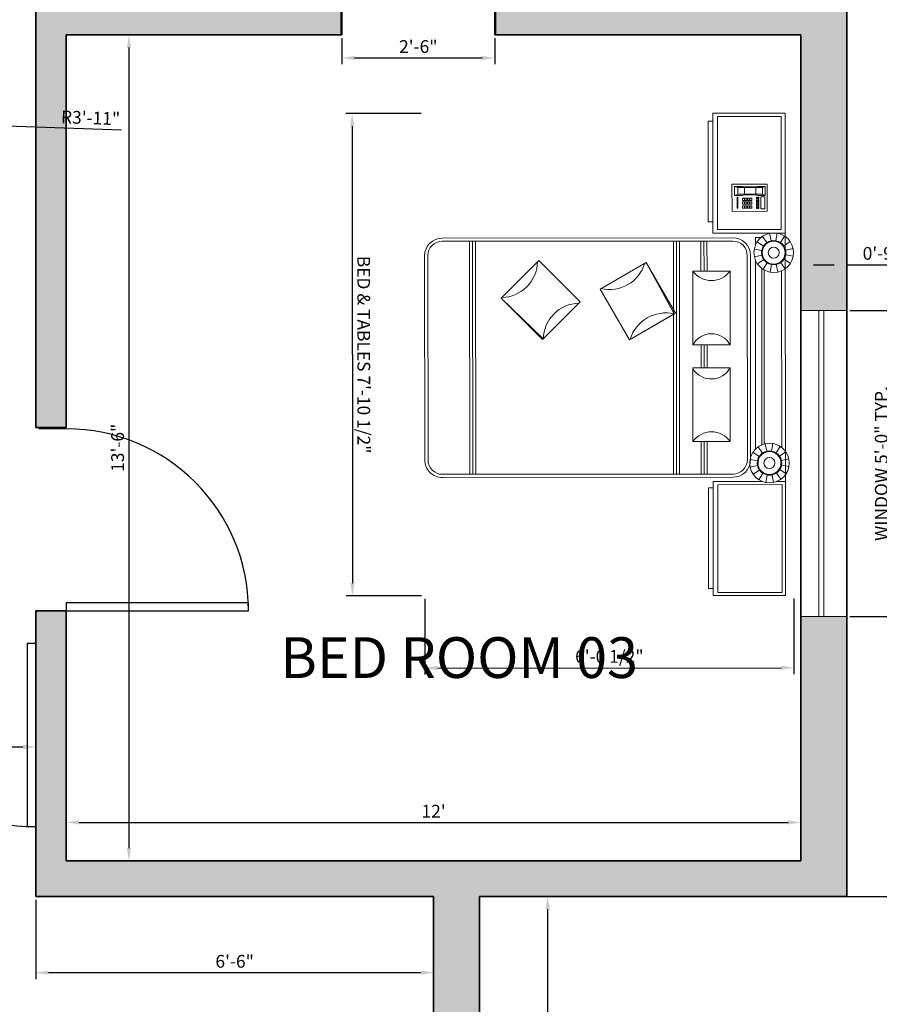
# Model space of a CAD drawing. Units: inches. Extents: x 2901 to 5923, y 918 to 2827.
# Tile 11 of 16: x 4730 to 4898, y 1227 to 1420. Entities that reach past the tile are written whole.
import ezdxf

# ---------------------------------------------------------------- set-up
doc = ezdxf.new("R2010")
doc.units = ezdxf.units.IN
for name, color, linetype, lineweight in [('A-ANNO-DIMS', 2, 'Continuous', 18), ('A-AREA-IDEN', 7, 'Continuous', 25), ('A-FLOR-PATT', 252, 'Continuous', 13), ('A-GLAZ', 4, 'Continuous', 18), ('A-WALL-PATT', 7, 'Continuous', 13), ('doors', 240, 'Continuous', 25), ('furniture', 160, 'Continuous', 18), ('walls', 7, 'Continuous', 35)]:
    doc.layers.add(name, color=color, linetype=linetype, lineweight=lineweight)
doc.styles.get("Standard").update_dxf_attribs({"font": 'arial.ttf'})
doc.dimstyles.new('Copy of ISO-25', dxfattribs={"dimtxt": 2.5, "dimasz": 2.5, "dimexe": 1.25, "dimexo": 0.625, "dimtad": 1, "dimdec": 1, "dimlunit": 4, "dimtxsty": 'Standard', "dimcen": 2.5, "dimadec": 0, "dimazin": 0, "dimtfac": 1, "dimtdec": 1, "dimtmove": 0, "dimatfit": 3, "dimfxl": 1, "dimarcsym": 0})

# ---------------------------------------------------------------- blocks, each defined once
blk = doc.blocks.new('*U9')
for p, q in [((-40, 0), (-40, 6)), ((0, 0), (0, 6))]:
    blk.add_line(p, q)
blk.add_lwpolyline([(0, 0), (0, -40), (-1.75, -40), (-1.75, 0)], close=True)
blk.add_arc((0, 0), 40, 180, 270)
blk = doc.blocks.new('*U7')
for p, q in [((0, 0), (0, 6)), ((40, 0), (40, 6))]:
    blk.add_line(p, q)
blk.add_lwpolyline([(0, 0), (0, -40), (1.75, -40), (1.75, 0)], close=True)
blk.add_arc((0, 0), 40, 270, 0)
blk = doc.blocks.new('*U2')
for p, q in [((0, 0), (0, -6)), ((40, 0), (40, -6))]:
    blk.add_line(p, q)
blk.add_lwpolyline([(0, 0), (0, 40), (1.75, 40), (1.75, 0)], close=True)
blk.add_arc((0, 0), 40, 0, 90)
blk = doc.blocks.new('A$C18EB7ED0')
for p, q in [((0.7653, 2.1814), (0.7911, 2.1442)), ((0.8076, 2.1998), (0.8172, 2.1555)), ((0.8537, 2.2006), (0.8456, 2.1559)), ((0.8966, 2.1836), (0.8721, 2.1455)), ((0, 2.1539), (2.8801, 2.1539)), ((0, 1.7209), (0, 2.1539)), ((0.0187, 2.129), (0.695, 2.129)), ((0.0187, 1.7489), (0.0187, 2.129)), ((0.695, 2.129), (0.695, 1.7489)), ((0.7156, 2.1539), (0.7156, 1.7209)), ((0.7332, 2.1483), (0.7713, 2.1237)), ((0.9298, 2.1515), (0.8925, 2.1257)), ((0.941, 2.1314), (1.9968, 2.1314)), ((1.9899, 2.1218), (2.028, 2.0973)), ((2.022, 2.155), (2.0478, 2.1177)), ((2.0643, 2.1733), (2.0739, 2.129)), ((2.1105, 2.1741), (2.1024, 2.1295)), ((2.1534, 2.1571), (2.1288, 2.119)), ((2.1865, 2.1251), (2.1493, 2.0992)), ((2.1997, 2.1), (2.1997, 2.1539)), ((2.2184, 2.1337), (2.8624, 2.1337)), ((2.2184, 1.7489), (2.2184, 2.1337)), ((2.8624, 2.1337), (2.8624, 1.7489)), ((2.8801, 2.1539), (2.8801, 1.7209)), ((0.7162, 2.1054), (0.7608, 2.0973)), ((0.717, 2.0593), (0.7613, 2.0688)), ((0.9481, 2.1092), (0.9038, 2.0996)), ((0.9489, 2.0631), (0.9043, 2.0712)), ((1.973, 2.0789), (2.0176, 2.0708)), ((2.2049, 2.0827), (2.1606, 2.0731)), ((0.5857, 2.0461), (0.4227, 2.0461)), ((0.4227, 2.0461), (0.4227, 1.8353)), ((0.4366, 2.0335), (0.4439, 2.018)), ((0.4903, 2.0335), (0.4366, 2.0335)), ((0.4366, 2.0335), (0.4366, 1.9902)), ((0.4824, 2.018), (0.4439, 2.018)), ((0.4824, 2.018), (0.4439, 2.018)), ((0.4439, 2.018), (0.4439, 1.8697)), ((0.4824, 2.018), (0.4903, 2.0335)), ((0.4824, 1.8697), (0.4824, 2.018)), ((0.4903, 1.9902), (0.4903, 2.0338)), ((0.5706, 2.0307), (0.4996, 2.0307)), ((0.4996, 2.0307), (0.4996, 2.0082)), ((0.4996, 2.0082), (0.5706, 2.0082)), ((0.5706, 2.0082), (0.5706, 2.0307)), ((0.5857, 1.8353), (0.5857, 2.0461)), ((0.7353, 2.0169), (0.7726, 2.0427)), ((0.7411, 2.0132), (0.7411, 1.9754)), ((0.7685, 1.9849), (0.7931, 2.023)), ((0.8114, 1.9679), (0.8195, 2.0125)), ((0.8575, 1.9687), (0.848, 2.013)), ((0.8999, 1.987), (0.8741, 2.0243)), ((0.9319, 2.0202), (0.8938, 2.0447)), ((1.9798, 2.0132), (0.9271, 2.0132)), ((1.9752, 2.0268), (0.9359, 2.0268)), ((1.9737, 2.0328), (2.0181, 2.0424)), ((1.9921, 1.9905), (2.0294, 2.0163)), ((2.1887, 1.9937), (2.1506, 2.0183)), ((2.2056, 2.0366), (2.161, 2.0447)), ((2.1997, 1.7209), (2.1997, 2.0155)), ((0.4366, 1.9902), (0.4391, 1.9789)), ((0.4391, 1.9789), (0.4391, 1.9067)), ((0.4824, 1.978), (0.4439, 1.978)), ((0.4903, 1.9902), (0.4871, 1.9789)), ((0.4871, 1.9789), (0.4871, 1.908)), ((0.514, 1.9963), (0.5013, 1.9963)), ((0.5013, 1.9963), (0.5013, 1.992)), ((0.5013, 1.992), (0.514, 1.992)), ((0.514, 1.9864), (0.5013, 1.9864)), ((0.5013, 1.9864), (0.5013, 1.9821)), ((0.5013, 1.9821), (0.514, 1.9821)), ((0.52, 1.9534), (0.5062, 1.9534)), ((0.5062, 1.9534), (0.5062, 1.9417)), ((0.5062, 1.9417), (0.52, 1.9417)), ((0.514, 1.992), (0.514, 1.9963)), ((0.514, 1.9821), (0.514, 1.9864)), ((0.5324, 1.9963), (0.5196, 1.9963)), ((0.5196, 1.9963), (0.5196, 1.992)), ((0.5196, 1.992), (0.5324, 1.992)), ((0.5324, 1.9864), (0.5196, 1.9864)), ((0.5196, 1.9864), (0.5196, 1.9821)), ((0.5196, 1.9821), (0.5324, 1.9821)), ((0.52, 1.9417), (0.52, 1.9534)), ((0.5426, 1.9534), (0.5288, 1.9534)), ((0.5288, 1.9534), (0.5288, 1.9417)), ((0.5288, 1.9417), (0.5426, 1.9417)), ((0.5324, 1.992), (0.5324, 1.9963)), ((0.5324, 1.9821), (0.5324, 1.9864)), ((0.5507, 1.9963), (0.538, 1.9963)), ((0.538, 1.9963), (0.538, 1.992)), ((0.538, 1.992), (0.5507, 1.992)), ((0.5507, 1.9864), (0.538, 1.9864)), ((0.538, 1.9864), (0.538, 1.9821)), ((0.538, 1.9821), (0.5507, 1.9821)), ((0.5426, 1.9417), (0.5426, 1.9534)), ((0.5507, 1.992), (0.5507, 1.9963)), ((0.5507, 1.9821), (0.5507, 1.9864)), ((0.5659, 1.9534), (0.5521, 1.9534)), ((0.5521, 1.9534), (0.5521, 1.9417)), ((0.5521, 1.9417), (0.5659, 1.9417)), ((0.5691, 1.9963), (0.5564, 1.9963)), ((0.5564, 1.9963), (0.5564, 1.992)), ((0.5564, 1.992), (0.5691, 1.992)), ((0.5691, 1.9864), (0.5564, 1.9864)), ((0.5564, 1.9864), (0.5564, 1.9821)), ((0.5564, 1.9821), (0.5691, 1.9821)), ((0.5659, 1.9417), (0.5659, 1.9534)), ((0.5691, 1.992), (0.5691, 1.9963)), ((0.5691, 1.9821), (0.5691, 1.9864)), ((0.7411, 1.9754), (0.7863, 1.9754)), ((2.0691, 1.9452), (0.8491, 1.9452)), ((0.8788, 1.9754), (2.0045, 1.9754)), ((2.0252, 1.9584), (2.0498, 1.9965)), ((2.0682, 1.9414), (2.0763, 1.986)), ((2.1143, 1.9422), (2.1047, 1.9865)), ((2.1566, 1.9605), (2.1308, 1.9978)), ((2.1742, 1.9754), (2.1771, 1.9754)), ((2.1771, 1.9754), (2.1771, 1.9785)), ((0.4391, 1.9067), (0.4366, 1.8971)), ((0.4366, 1.8971), (0.4366, 1.8504)), ((0.4439, 1.9101), (0.4824, 1.9101)), ((0.4871, 1.908), (0.4903, 1.8971)), ((0.4903, 1.8499), (0.4903, 1.8971)), ((0.52, 1.9385), (0.5062, 1.9385)), ((0.5062, 1.9385), (0.5062, 1.9269)), ((0.5062, 1.9269), (0.52, 1.9269)), ((0.52, 1.9237), (0.5062, 1.9237)), ((0.5062, 1.9237), (0.5062, 1.9121)), ((0.5062, 1.9121), (0.52, 1.9121)), ((0.52, 1.9089), (0.5062, 1.9089)), ((0.5062, 1.9089), (0.5062, 1.8972)), ((0.5062, 1.8972), (0.52, 1.8972)), ((0.52, 1.9269), (0.52, 1.9385)), ((0.52, 1.9121), (0.52, 1.9237)), ((0.52, 1.8972), (0.52, 1.9089)), ((0.5426, 1.9385), (0.5288, 1.9385)), ((0.5288, 1.9385), (0.5288, 1.9269)), ((0.5288, 1.9269), (0.5426, 1.9269)), ((0.5426, 1.9237), (0.5288, 1.9237)), ((0.5288, 1.9237), (0.5288, 1.9121)), ((0.5288, 1.9121), (0.5426, 1.9121)), ((0.5426, 1.9089), (0.5288, 1.9089)), ((0.5288, 1.9089), (0.5288, 1.8972)), ((0.5288, 1.8972), (0.5426, 1.8972)), ((0.5426, 1.9269), (0.5426, 1.9385)), ((0.5426, 1.9121), (0.5426, 1.9237)), ((0.5426, 1.8972), (0.5426, 1.9089)), ((0.5659, 1.9385), (0.5521, 1.9385)), ((0.5521, 1.9385), (0.5521, 1.9269)), ((0.5521, 1.9269), (0.5659, 1.9269)), ((0.5659, 1.9237), (0.5521, 1.9237)), ((0.5521, 1.9237), (0.5521, 1.9121)), ((0.5521, 1.9121), (0.5659, 1.9121)), ((0.5659, 1.9089), (0.5521, 1.9089)), ((0.5521, 1.9089), (0.5521, 1.8972)), ((0.5521, 1.8972), (0.5659, 1.8972)), ((0.5659, 1.9269), (0.5659, 1.9385)), ((0.5659, 1.9121), (0.5659, 1.9237)), ((0.5659, 1.8972), (0.5659, 1.9089)), ((2.0691, 1.926), (0.8491, 1.926)), ((0.4227, 1.8353), (0.5857, 1.8353)), ((0.4439, 1.8697), (0.4366, 1.8504)), ((0.4366, 1.8504), (0.4903, 1.8504)), ((0.4824, 1.8697), (0.4439, 1.8697)), ((0.4439, 1.8697), (0.4824, 1.8697)), ((0.4903, 1.8504), (0.4824, 1.8697)), ((0.5208, 1.8697), (0.5009, 1.8697)), ((0.5009, 1.8697), (0.5009, 1.8657)), ((0.5009, 1.8657), (0.5208, 1.8657)), ((0.5208, 1.8657), (0.5208, 1.8697)), ((0.5433, 1.8697), (0.5234, 1.8697)), ((0.5234, 1.8697), (0.5234, 1.8657)), ((0.5234, 1.8657), (0.5433, 1.8657)), ((0.5433, 1.8657), (0.5433, 1.8697)), ((0.5658, 1.8697), (0.546, 1.8697)), ((0.546, 1.8697), (0.546, 1.8657)), ((0.546, 1.8657), (0.5658, 1.8657)), ((0.5658, 1.8657), (0.5658, 1.8697)), ((0.7439, 1.8401), (0.7439, 0.1052)), ((0.7632, 1.8401), (0.7632, 0.1052)), ((2.155, 0.1052), (2.155, 1.8401)), ((2.1743, 0.1052), (2.1743, 1.8401)), ((0.9429, 1.8231), (1.3829, 1.8231)), ((0.9429, 1.601), (0.9429, 1.8231)), ((1.3829, 1.8231), (1.3829, 1.601)), ((1.5207, 1.601), (1.5207, 1.8231)), ((1.5207, 1.8231), (1.9608, 1.8231)), ((1.9608, 1.8231), (1.9608, 1.601)), ((0.7156, 1.7209), (0, 1.7209)), ((0, 1.7209), (0.6483, 1.7209)), ((0.695, 1.7489), (0.0187, 1.7489)), ((0.0462, 1.6929), (0.0462, 1.7209)), ((0.6483, 1.7209), (0.6483, 1.6929)), ((2.8801, 1.7209), (2.1997, 1.7209)), ((2.8624, 1.7489), (2.2184, 1.7489)), ((2.2369, 1.7209), (2.8801, 1.7209)), ((2.2369, 1.6929), (2.2369, 1.7209)), ((2.839, 1.7209), (2.839, 1.6929)), ((0.6483, 1.6929), (0.0462, 1.6929)), ((0.7632, 1.6858), (0.9429, 1.6858)), ((0.7632, 1.6678), (0.9429, 1.6678)), ((0.7632, 1.6498), (0.9429, 1.6498)), ((1.3829, 1.6858), (1.5207, 1.6858)), ((1.3829, 1.6678), (1.5207, 1.6678)), ((1.3829, 1.6498), (1.5207, 1.6498)), ((1.9608, 1.6858), (2.155, 1.6858)), ((1.9608, 1.6678), (2.155, 1.6678)), ((1.9608, 1.6498), (2.155, 1.6498)), ((2.839, 1.6929), (2.2369, 1.6929)), ((1.3829, 1.601), (0.9429, 1.601)), ((1.9608, 1.601), (1.5207, 1.601)), ((0.7632, 1.5215), (2.155, 1.5215)), ((0.7632, 1.5035), (2.155, 1.5035)), ((0.7632, 1.4855), (2.155, 1.4855)), ((0.8904, 1.3226), (1.1935, 1.4976)), ((0.8904, 1.3226), (1.1982, 1.4894)), ((1.1935, 1.4976), (1.3524, 1.2224)), ((1.1982, 1.4894), (1.3524, 1.2224)), ((1.0493, 1.0474), (0.8904, 1.3226)), ((1.0493, 1.0474), (0.8904, 1.3226)), ((1.3524, 1.2224), (1.0493, 1.0474)), ((1.3524, 1.2224), (1.0493, 1.0474)), ((0.8789, 0.6811), (1.1264, 0.9286)), ((0.8789, 0.6811), (1.1264, 0.9286)), ((1.1264, 0.9286), (1.3473, 0.7077)), ((1.1264, 0.9286), (1.3511, 0.7039)), ((1.3473, 0.7077), (1.1036, 0.4564)), ((1.1036, 0.4564), (0.8789, 0.6811)), ((1.1036, 0.4564), (0.8789, 0.6811)), ((1.3511, 0.7039), (1.1036, 0.4564)), ((0.7632, 0.3045), (2.155, 0.3045)), ((0.7632, 0.2865), (2.155, 0.2865)), ((0.7632, 0.2685), (2.155, 0.2685)), ((0.8491, 0.0193), (2.0691, 0.0193)), ((0.8491, 0), (2.0691, 0))]:
    blk.add_line(p, q)
for centre, radius in [((0.8326, 2.0842), 0.1182), ((0.8326, 2.0842), 0.0729), ((0.8326, 2.0842), 0.0684), ((2.0893, 2.0578), 0.1182), ((2.0893, 2.0578), 0.0729), ((2.0893, 2.0578), 0.0684), ((0.8326, 2.0842), 0.0328), ((2.0893, 2.0578), 0.0328)]:
    blk.add_circle(centre, radius)
for centre, radius, start, end in [((0.8491, 1.8401), 0.1052, 90, 180), ((2.0691, 1.8401), 0.1052, 0, 90), ((0.8491, 1.8401), 0.0859, 90, 180), ((2.0691, 1.8401), 0.0859, 0, 90), ((0.8604, 1.712), 0.1383, 306.59595, 53.40405), ((1.4431, 1.712), 0.1263, 118.46186, 241.53814), ((1.4584, 1.7106), 0.1286, 303.40233, 61.02638), ((2.0371, 1.712), 0.1347, 124.50267, 235.49733), ((1.4126, 1.4383), 0.2204, 166.58792, 253.41208), ((0.8322, 1.1031), 0.2204, 346.58792, 73.41208), ((1.3534, 0.928), 0.2204, 181.58792, 268.41208), ((0.8795, 0.4541), 0.2204, 1.58792, 88.41208), ((0.8491, 0.1052), 0.1052, 180, 270), ((0.8491, 0.1052), 0.0859, 180, 270), ((2.0691, 0.1052), 0.1052, 270, 0), ((2.0691, 0.1052), 0.0859, 270, 0)]:
    blk.add_arc(centre, radius, start, end)
blk = doc.blocks.new('*D34')
at = {"layer": 'A-ANNO-DIMS', "color": 0, "lineweight": -2, "transparency": 16777216}
for p, q in [((4820.69, 1248.4), (4834.68, 1248.4)), ((4833.43, 1145.9), (4833.43, 1245.9)), ((4820.69, 1143.4), (4834.68, 1143.4))]:
    blk.add_line(p, q, dxfattribs=at)
at = {"layer": 'A-ANNO-DIMS', "color": 0, "transparency": 16777216}
for points in [[(4833.01, 1245.9), (4833.85, 1245.9), (4833.43, 1248.4)], [(4833.01, 1145.9), (4833.85, 1145.9), (4833.43, 1143.4)]]:
    blk.add_solid(points, dxfattribs=at)
at = {"layer": 'Defpoints', "color": 0, "transparency": 16777216}
for p in [(4820.07, 1248.4), (4833.43, 1248.4), (4820.07, 1143.4)]:
    blk.add_point(p, dxfattribs=at)
at = {"layer": 'A-ANNO-DIMS', "color": 0, "transparency": 16777216, "insert": (4831.53, 1195.9), "char_height": 2.5, "attachment_point": 5, "rotation": 90}
blk.add_mtext('8\'-9"', dxfattribs=at)
blk = doc.blocks.new('*D35')
at = {"layer": 'A-ANNO-DIMS', "color": 0, "lineweight": -2, "transparency": 16777216}
for p, q in [((4892.69, 1630.4), (4902.74, 1630.4)), ((4901.49, 1250.9), (4901.49, 1627.9)), ((4892.69, 1248.4), (4902.74, 1248.4))]:
    blk.add_line(p, q, dxfattribs=at)
at = {"layer": 'A-ANNO-DIMS', "color": 0, "transparency": 16777216}
for points in [[(4901.07, 1627.9), (4901.91, 1627.9), (4901.49, 1630.4)], [(4901.07, 1250.9), (4901.91, 1250.9), (4901.49, 1248.4)]]:
    blk.add_solid(points, dxfattribs=at)
at = {"layer": 'Defpoints', "color": 0, "transparency": 16777216}
for p in [(4892.07, 1630.4), (4901.49, 1630.4), (4892.07, 1248.4)]:
    blk.add_point(p, dxfattribs=at)
at = {"layer": 'A-ANNO-DIMS', "color": 0, "transparency": 16777216, "insert": (4899.59, 1439.4), "char_height": 2.5, "attachment_point": 5, "rotation": 90}
blk.add_mtext('31\'-10"', dxfattribs=at)
blk = doc.blocks.new('*D60')
at = {"layer": 'A-ANNO-DIMS', "color": 0, "lineweight": -2, "transparency": 16777216}
for p, q in [((4793.07, 1416.77), (4793.07, 1411.61)), ((4823.07, 1416.77), (4823.07, 1411.61)), ((4795.57, 1412.86), (4820.57, 1412.86))]:
    blk.add_line(p, q, dxfattribs=at)
at = {"layer": 'A-ANNO-DIMS', "color": 0, "transparency": 16777216}
for points in [[(4795.57, 1413.28), (4795.57, 1412.45), (4793.07, 1412.86)], [(4820.57, 1413.28), (4820.57, 1412.45), (4823.07, 1412.86)]]:
    blk.add_solid(points, dxfattribs=at)
at = {"layer": 'Defpoints', "color": 0, "transparency": 16777216}
for p in [(4793.07, 1417.4), (4823.07, 1417.4), (4823.07, 1412.86)]:
    blk.add_point(p, dxfattribs=at)
at = {"layer": 'A-ANNO-DIMS', "color": 0, "transparency": 16777216, "insert": (4808.07, 1414.77), "char_height": 2.5, "attachment_point": 5}
blk.add_mtext('2\'-6"', dxfattribs=at)
blk = doc.blocks.new('*D62')
at = {"layer": 'A-ANNO-DIMS', "color": 0, "lineweight": -2, "transparency": 16777216}
for p, q in [((4589.07, 1296.77), (4589.07, 1276.48)), ((4733.07, 1296.77), (4733.07, 1276.48)), ((4591.57, 1277.73), (4730.57, 1277.73))]:
    blk.add_line(p, q, dxfattribs=at)
at = {"layer": 'A-ANNO-DIMS', "color": 0, "transparency": 16777216}
for points in [[(4591.57, 1278.14), (4591.57, 1277.31), (4589.07, 1277.73)], [(4730.57, 1278.14), (4730.57, 1277.31), (4733.07, 1277.73)]]:
    blk.add_solid(points, dxfattribs=at)
at = {"layer": 'Defpoints', "color": 0, "transparency": 16777216}
for p in [(4589.07, 1297.4), (4733.07, 1297.4), (4733.07, 1277.73)]:
    blk.add_point(p, dxfattribs=at)
at = {"layer": 'A-ANNO-DIMS', "color": 0, "transparency": 16777216, "insert": (4661.07, 1279.61), "char_height": 2.5, "attachment_point": 5}
blk.add_mtext("12'", dxfattribs=at)
blk = doc.blocks.new('*D63')
at = {"layer": 'A-ANNO-DIMS', "color": 0, "lineweight": -2, "transparency": 16777216}
for p, q in [((4733.07, 1247.77), (4733.07, 1232.21)), ((4811.07, 1247.77), (4811.07, 1232.21)), ((4735.57, 1233.46), (4808.57, 1233.46))]:
    blk.add_line(p, q, dxfattribs=at)
at = {"layer": 'A-ANNO-DIMS', "color": 0, "transparency": 16777216}
for points in [[(4735.57, 1233.88), (4735.57, 1233.04), (4733.07, 1233.46)], [(4808.57, 1233.88), (4808.57, 1233.04), (4811.07, 1233.46)]]:
    blk.add_solid(points, dxfattribs=at)
at = {"layer": 'Defpoints', "color": 0, "transparency": 16777216}
for p in [(4733.07, 1248.4), (4811.07, 1248.4), (4811.07, 1233.46)]:
    blk.add_point(p, dxfattribs=at)
at = {"layer": 'A-ANNO-DIMS', "color": 0, "transparency": 16777216, "insert": (4772.07, 1235.36), "char_height": 2.5, "attachment_point": 5}
blk.add_mtext('6\'-6"', dxfattribs=at)
blk = doc.blocks.new('*D64')
at = {"layer": 'A-ANNO-DIMS', "color": 0, "lineweight": -2, "transparency": 16777216}
for p, q in [((4739.07, 1256.02), (4739.07, 1264.17)), ((4883.07, 1256.02), (4883.07, 1264.17)), ((4741.57, 1262.92), (4880.57, 1262.92))]:
    blk.add_line(p, q, dxfattribs=at)
at = {"layer": 'A-ANNO-DIMS', "color": 0, "transparency": 16777216}
for points in [[(4741.57, 1263.34), (4741.57, 1262.5), (4739.07, 1262.92)], [(4880.57, 1263.34), (4880.57, 1262.5), (4883.07, 1262.92)]]:
    blk.add_solid(points, dxfattribs=at)
at = {"layer": 'Defpoints', "color": 0, "transparency": 16777216}
for p in [(4883.07, 1262.92), (4739.07, 1255.4), (4883.07, 1255.4)]:
    blk.add_point(p, dxfattribs=at)
at = {"layer": 'A-ANNO-DIMS', "color": 0, "transparency": 16777216, "insert": (4811.07, 1264.8), "char_height": 2.5, "attachment_point": 5}
blk.add_mtext("12'", dxfattribs=at)
blk = doc.blocks.new('*D65')
at = {"layer": 'A-ANNO-DIMS', "color": 0, "lineweight": -2, "transparency": 16777216}
for p, q in [((4739.69, 1417.4), (4752.6, 1417.4)), ((4751.35, 1414.9), (4751.35, 1257.9)), ((4739.69, 1255.4), (4752.6, 1255.4))]:
    blk.add_line(p, q, dxfattribs=at)
at = {"layer": 'A-ANNO-DIMS', "color": 0, "transparency": 16777216}
for points in [[(4750.94, 1414.9), (4751.77, 1414.9), (4751.35, 1417.4)], [(4750.94, 1257.9), (4751.77, 1257.9), (4751.35, 1255.4)]]:
    blk.add_solid(points, dxfattribs=at)
at = {"layer": 'Defpoints', "color": 0, "transparency": 16777216}
for p in [(4739.07, 1417.4), (4739.07, 1255.4), (4751.35, 1255.4)]:
    blk.add_point(p, dxfattribs=at)
at = {"layer": 'A-ANNO-DIMS', "color": 0, "transparency": 16777216, "insert": (4749.45, 1336.4), "char_height": 2.5, "attachment_point": 5, "rotation": 90}
blk.add_mtext('13\'-6"', dxfattribs=at)
blk = doc.blocks.new('WIN-60')
for p, q in [((60, 9), (0, 9)), ((0, 9), (0, 0)), ((60, 0), (60, 9)), ((0, 4.5), (60, 4.5)), ((0, 3.5), (60, 3.5))]:
    blk.add_line(p, q)
blk = doc.blocks.new('*D73')
at = {"layer": 'A-ANNO-DIMS', "color": 0, "lineweight": -2, "transparency": 16777216}
for p, q in [((4892.69, 1363.31), (4902.32, 1363.31)), ((4901.07, 1360.81), (4901.07, 1305.81)), ((4892.69, 1303.31), (4902.32, 1303.31))]:
    blk.add_line(p, q, dxfattribs=at)
at = {"layer": 'A-ANNO-DIMS', "color": 0, "transparency": 16777216}
for points in [[(4900.65, 1360.81), (4901.49, 1360.81), (4901.07, 1363.31)], [(4900.65, 1305.81), (4901.49, 1305.81), (4901.07, 1303.31)]]:
    blk.add_solid(points, dxfattribs=at)
at = {"layer": 'Defpoints', "color": 0, "transparency": 16777216}
for p in [(4892.07, 1363.31), (4892.07, 1303.31), (4901.07, 1303.31)]:
    blk.add_point(p, dxfattribs=at)
at = {"layer": 'A-ANNO-DIMS', "color": 0, "transparency": 16777216, "insert": (4899.15, 1333.31), "char_height": 2.5, "attachment_point": 5, "rotation": 90}
blk.add_mtext('WINDOW 5\'-0" TYP.', dxfattribs=at)
blk = doc.blocks.new('*D74')
at = {"layer": 'A-ANNO-DIMS', "color": 0, "lineweight": -2, "transparency": 16777216}
for p, q in [((4883.07, 1363.93), (4883.07, 1373.56)), ((4892.07, 1363.93), (4892.07, 1373.56)), ((4885.57, 1372.31), (4889.57, 1372.31)), ((4892.07, 1372.31), (4911.06, 1372.31))]:
    blk.add_line(p, q, dxfattribs=at)
at = {"layer": 'A-ANNO-DIMS', "color": 0, "transparency": 16777216}
for points in [[(4885.57, 1372.72), (4885.57, 1371.89), (4883.07, 1372.31)], [(4889.57, 1372.72), (4889.57, 1371.89), (4892.07, 1372.31)]]:
    blk.add_solid(points, dxfattribs=at)
at = {"layer": 'Defpoints', "color": 0, "transparency": 16777216}
for p in [(4892.07, 1372.31), (4883.07, 1363.31), (4892.07, 1363.31)]:
    blk.add_point(p, dxfattribs=at)
at = {"layer": 'A-ANNO-DIMS', "color": 0, "transparency": 16777216, "insert": (4902.81, 1374.21), "char_height": 2.5, "attachment_point": 5}
blk.add_mtext('0\'-9" TYP.', dxfattribs=at)
blk = doc.blocks.new('*D87')
at = {"layer": 'A-ANNO-DIMS', "color": 0, "lineweight": -2, "transparency": 16777216}
for p, q in [((4808.66, 1401.96), (4793.85, 1401.95)), ((4795.1, 1399.45), (4795.17, 1309.88)), ((4808.73, 1307.39), (4793.92, 1307.38))]:
    blk.add_line(p, q, dxfattribs=at)
at = {"layer": 'A-ANNO-DIMS', "color": 0, "transparency": 16777216}
for points in [[(4795.52, 1399.45), (4794.69, 1399.45), (4795.1, 1401.95)], [(4795.59, 1309.88), (4794.75, 1309.88), (4795.17, 1307.38)]]:
    blk.add_solid(points, dxfattribs=at)
at = {"layer": 'Defpoints', "color": 0, "transparency": 16777216}
for p in [(4809.29, 1401.96), (4795.17, 1307.38), (4809.36, 1307.39)]:
    blk.add_point(p, dxfattribs=at)
at = {"layer": 'A-ANNO-DIMS', "color": 0, "transparency": 16777216, "insert": (4797.06, 1354.67), "char_height": 2.5, "attachment_point": 5, "rotation": 270.0422}
blk.add_mtext('BED & TABLES 7\'-10 1/2"', dxfattribs=at)
blk = doc.blocks.new('*D88')
at = {"layer": 'A-ANNO-DIMS', "color": 0, "lineweight": -2, "transparency": 16777216}
for p, q in [((4809.36, 1306.77), (4809.37, 1291.96)), ((4881.68, 1306.82), (4881.69, 1292.01)), ((4811.87, 1293.21), (4879.19, 1293.26))]:
    blk.add_line(p, q, dxfattribs=at)
at = {"layer": 'A-ANNO-DIMS', "color": 0, "transparency": 16777216}
for points in [[(4811.87, 1293.63), (4811.87, 1292.79), (4809.37, 1293.21)], [(4879.19, 1293.67), (4879.19, 1292.84), (4881.69, 1293.26)]]:
    blk.add_solid(points, dxfattribs=at)
at = {"layer": 'Defpoints', "color": 0, "transparency": 16777216}
for p in [(4809.36, 1307.39), (4881.68, 1307.45), (4881.69, 1293.26)]:
    blk.add_point(p, dxfattribs=at)
at = {"layer": 'A-ANNO-DIMS', "color": 0, "transparency": 16777216, "insert": (4845.52, 1295.15), "char_height": 2.5, "attachment_point": 5, "rotation": 0.0422}
blk.add_mtext('6\'-0 1/2"', dxfattribs=at)
blk = doc.blocks.new('*D89')
at = {"layer": 'A-ANNO-DIMS', "color": 0, "lineweight": -2, "transparency": 16777216}
for p, q in [((4892.69, 1630.4), (5055.73, 1630.4)), ((5054.48, 989.9), (5054.48, 1627.9)), ((4709.69, 987.4), (5055.73, 987.4))]:
    blk.add_line(p, q, dxfattribs=at)
at = {"layer": 'A-ANNO-DIMS', "color": 0, "transparency": 16777216}
for points in [[(5054.06, 1627.9), (5054.9, 1627.9), (5054.48, 1630.4)], [(5054.06, 989.9), (5054.9, 989.9), (5054.48, 987.4)]]:
    blk.add_solid(points, dxfattribs=at)
at = {"layer": 'Defpoints', "color": 0, "transparency": 16777216}
for p in [(4892.07, 1630.4), (5054.48, 1630.4), (4709.07, 987.4)]:
    blk.add_point(p, dxfattribs=at)
at = {"layer": 'A-ANNO-DIMS', "color": 0, "transparency": 16777216, "insert": (5052.58, 1308.9), "char_height": 2.5, "attachment_point": 5, "rotation": 90}
blk.add_mtext('53\'-7"', dxfattribs=at)
blk = doc.blocks.new('*D97')
at = {"layer": 'A-ANNO-DIMS', "color": 0, "lineweight": -2, "transparency": 16777216}
for p, q in [((4892.69, 1458.87), (5055.73, 1458.87)), ((5054.48, 1456.37), (5054.48, 1365.81)), ((4892.69, 1363.31), (5055.73, 1363.31))]:
    blk.add_line(p, q, dxfattribs=at)
at = {"layer": 'A-ANNO-DIMS', "color": 0, "transparency": 16777216}
for points in [[(5054.06, 1456.37), (5054.9, 1456.37), (5054.48, 1458.87)], [(5054.06, 1365.81), (5054.9, 1365.81), (5054.48, 1363.31)]]:
    blk.add_solid(points, dxfattribs=at)
at = {"layer": 'Defpoints', "color": 0, "transparency": 16777216}
for p in [(4892.07, 1458.87), (4892.07, 1363.31), (5054.48, 1363.31)]:
    blk.add_point(p, dxfattribs=at)
at = {"layer": 'A-ANNO-DIMS', "color": 0, "transparency": 16777216, "insert": (5052.56, 1411.09), "char_height": 2.5, "attachment_point": 5, "rotation": 90}
blk.add_mtext('7\'-11 1/2"', dxfattribs=at)
blk = doc.blocks.new('*D99')
at = {"layer": 'A-ANNO-DIMS', "color": 0, "lineweight": -2, "transparency": 16777216}
for p, q in [((4820.69, 1248.4), (5055.73, 1248.4)), ((5054.48, 1214.66), (5054.48, 1245.9)), ((4820.69, 1212.16), (5055.73, 1212.16))]:
    blk.add_line(p, q, dxfattribs=at)
at = {"layer": 'A-ANNO-DIMS', "color": 0, "transparency": 16777216}
for points in [[(5054.06, 1245.9), (5054.9, 1245.9), (5054.48, 1248.4)], [(5054.06, 1214.66), (5054.9, 1214.66), (5054.48, 1212.16)]]:
    blk.add_solid(points, dxfattribs=at)
at = {"layer": 'Defpoints', "color": 0, "transparency": 16777216}
for p in [(4820.07, 1248.4), (5054.48, 1248.4), (4820.07, 1212.16)]:
    blk.add_point(p, dxfattribs=at)
at = {"layer": 'A-ANNO-DIMS', "color": 0, "transparency": 16777216, "insert": (5052.58, 1230.28), "char_height": 2.5, "attachment_point": 5, "rotation": 90}
blk.add_mtext('3\'-0"', dxfattribs=at)
blk = doc.blocks.new('*D108')
at = {"layer": 'A-ANNO-DIMS', "color": 0, "lineweight": -2, "transparency": 16777216}
for p, q in [((4668.21, 1401.5), (4715.42, 1399.87)), ((4749.86, 1398.67), (4717.92, 1399.78))]:
    blk.add_line(p, q, dxfattribs=at)
at = {"layer": 'A-ANNO-DIMS', "color": 0, "transparency": 16777216}
blk.add_solid([(4717.94, 1400.2), (4717.91, 1399.36), (4715.42, 1399.87)], dxfattribs=at)
at = {"layer": 'Defpoints', "color": 0, "transparency": 16777216}
for p in [(4668.21, 1401.5), (4715.42, 1399.87)]:
    blk.add_point(p, dxfattribs=at)
at = {"layer": 'A-ANNO-DIMS', "color": 0, "transparency": 16777216, "insert": (4743.82, 1400.79), "char_height": 2.5, "attachment_point": 5, "rotation": 358.0189}
blk.add_mtext('R3\'-11"', dxfattribs=at)

msp = doc.modelspace()

# ---------------------------------------------------------------- hatches: boundary and pattern name
at = {"layer": 'A-FLOR-PATT'}
h = msp.add_hatch(dxfattribs=at)
h.set_pattern_fill('ANSI32', color=256)
h.paths.add_polyline_path([(4883.07, 1621.4), (4739.07, 1621.4), (4739.07, 1564.39, -0.396616), (4774.43, 1529.97), (4774.46, 1529.97), (4774.46, 1528.4), (4883.07, 1528.4)])
h.paths.add_polyline_path([(4733.07, 1143.4), (4685.07, 1143.4), (4685.07, 1147.03), (4684.01, 1147.03), (4684.01, 1171.22, 0.413071), (4660.87, 1146.06, 0.412532), (4638.11, 1170.77), (4638.11, 1146.97), (4637.07, 1143.4), (4589.07, 1143.4), (4589.07, 1029.4), (4733.07, 1029.4)])
h.paths.add_polyline_path([(4620.35, 1086.26, -0.333335), (4622.56, 1084.04), (4622.56, 1084.04), (4712.62, 1084.04, -0.333335), (4714.84, 1086.26), (4718.53, 1086.26, -0.376086), (4721.48, 1084.04), (4721.48, 1062.64), (4721.48, 1041.23, -0.333387), (4718.96, 1039.01), (4714.84, 1039.01, -0.333335), (4712.62, 1041.23), (4712.62, 1041.23), (4622.56, 1041.23, -0.333335), (4620.35, 1039.01), (4616.66, 1039.01, -0.376086), (4613.71, 1041.23), (4613.71, 1062.63), (4613.71, 1084.04, -0.333387), (4616.23, 1086.26)], flags=16)
h.paths.add_polyline_path([(4638.8, 1084.04), (4643.23, 1078.14), (4678.67, 1078.14), (4687.53, 1084.04), (4687.53, 1071.49), (4718.53, 1067.06), (4718.53, 1062.64), (4718.53, 1058.21), (4687.53, 1053.78), (4687.53, 1041.23), (4678.67, 1047.13), (4643.23, 1047.13), (4638.8, 1041.23), (4638.8, 1062.63)], flags=0)
at = {"layer": 'A-WALL-PATT'}
h = msp.add_hatch(color=256, dxfattribs=at)
h.dxf.hatch_style = 1
h.paths.add_polyline_path([(4439.07, 1447.4), (4583.07, 1447.4), (4583.07, 1340.4), (4589.07, 1340.4), (4589.07, 1453.4), (4589.07, 1455.39), (4583.07, 1455.39), (4583.07, 1453.4), (4439.07, 1453.4), (4439.07, 1501.84), (4430.07, 1501.84), (4430.07, 1399.4), (4439.07, 1399.4)])
h.paths.add_polyline_path([(4439.07, 1621.4), (4487.07, 1621.4), (4487.07, 1630.4), (4430.07, 1630.4), (4430.07, 1561.84), (4439.07, 1561.84)])
h.paths.add_polyline_path([(4630.61, 1630.4), (4535.07, 1630.4), (4535.07, 1621.4), (4583.07, 1621.4), (4583.07, 1495.4), (4589.07, 1495.4), (4637.07, 1495.4), (4637.07, 1501.4), (4589.07, 1501.4), (4589.07, 1621.4), (4630.61, 1621.4)])
h.paths.add_polyline_path([(4892.07, 1630.4), (4690.61, 1630.4), (4690.61, 1621.4), (4733.07, 1621.4), (4733.07, 1564.4), (4739.07, 1564.4), (4739.07, 1621.4), (4883.07, 1621.4), (4883.07, 1528.4), (4739.07, 1528.4), (4733.07, 1528.4), (4733.07, 1501.4), (4685.07, 1501.4), (4685.07, 1495.4), (4739.07, 1495.4), (4739.07, 1519.4), (4787.07, 1519.4), (4787.07, 1423.4), (4739.07, 1423.4), (4739.07, 1456.67), (4733.07, 1456.67), (4733.07, 1340.4), (4739.07, 1340.4), (4739.07, 1417.4), (4787.07, 1417.4), (4793.07, 1417.4), (4793.07, 1423.4), (4793.07, 1519.4), (4883.07, 1519.4), (4883.07, 1482.87), (4892.07, 1482.87)])
h.paths.add_polyline_path([(4892.07, 1458.87), (4883.07, 1458.87), (4883.07, 1423.4), (4823.07, 1423.4), (4823.07, 1417.4), (4883.07, 1417.4), (4883.07, 1363.31), (4892.07, 1363.31)], flags=17)
h.paths.add_polyline_path([(4892.07, 1303.31), (4883.07, 1303.31), (4883.07, 1255.4), (4739.07, 1255.4), (4739.07, 1304.4), (4733.07, 1304.4), (4733.07, 1303.4), (4733.07, 1297.4), (4733.07, 1255.4), (4733.07, 1248.4), (4811.07, 1248.4), (4811.07, 1212.16), (4820.07, 1212.16), (4820.07, 1248.4), (4892.07, 1248.4)])
h.paths.add_polyline_path([(4820.07, 1182.16), (4811.07, 1182.16), (4811.07, 1152.4), (4685.07, 1152.4), (4685.07, 1147.03), (4685.07, 1143.4), (4733.07, 1143.4), (4811.07, 1143.4), (4814.07, 1143.4), (4820.07, 1143.4)])
h.paths.add_polyline_path([(4637.07, 1152.4), (4589.07, 1152.4), (4589.07, 1153.4), (4583.86, 1153.4), (4583.07, 1153.4), (4583.07, 1152.4), (4511.07, 1152.4), (4511.07, 1182.16), (4502.07, 1182.16), (4502.07, 1143.4), (4568.07, 1143.4), (4583.07, 1143.4), (4583.07, 1023.4), (4739.07, 1023.4), (4739.07, 1143.4), (4733.07, 1143.4), (4733.07, 1029.4), (4589.07, 1029.4), (4589.07, 1143.4), (4637.07, 1143.4), (4637.07, 1146.97)])
h.paths.add_polyline_path([(4511.07, 1246.4), (4583.07, 1246.4), (4583.07, 1188.4), (4589.07, 1188.4), (4589.07, 1246.4), (4589.07, 1248.4), (4589.07, 1255.4), (4589.07, 1297.4), (4697.07, 1297.4), (4697.07, 1303.4), (4589.07, 1303.4), (4589.07, 1304.4), (4583.07, 1304.4), (4583.07, 1255.4), (4439.07, 1255.4), (4439.07, 1261.4), (4439.07, 1351.4), (4430.07, 1351.4), (4430.07, 1252.4), (4430.07, 1246.4), (4439.07, 1246.4), (4487.07, 1246.4), (4502.07, 1246.4), (4502.07, 1212.16), (4511.07, 1212.16)])

# ---------------------------------------------------------------- linework, layer by layer
at = {"layer": 'walls'}
for p, q in [((4892.07, 1630.4), (4892.07, 1248.4)), ((4733.07, 1456.67), (4733.07, 1340.4)), ((4793.07, 1423.4), (4793.07, 1417.4)), ((4823.07, 1423.4), (4823.07, 1417.4)), ((4787.07, 1417.4), (4739.07, 1417.4)), ((4739.07, 1340.4), (4739.07, 1417.4)), ((4787.07, 1417.4), (4793.07, 1417.4)), ((4793.07, 1417.4), (4792.85, 1417.4)), ((4823.07, 1417.4), (4883.07, 1417.4)), ((4883.07, 1417.4), (4883.07, 1255.4)), ((4883.07, 1417.4), (4883.07, 1363.31)), ((4739.07, 1340.4), (4733.07, 1340.4)), ((4733.07, 1303.4), (4733.07, 1304.4)), ((4733.07, 1304.4), (4739.07, 1304.4)), ((4733.07, 1304.4), (4733.07, 1303.4)), ((4739.07, 1255.4), (4739.07, 1304.4)), ((4733.07, 1303.4), (4733.07, 1297.4)), ((4733.07, 1297.4), (4733.07, 1255.4)), ((4733.07, 1255.4), (4733.07, 1248.4)), ((4739.07, 1255.4), (4883.07, 1255.4)), ((4733.07, 1248.4), (4811.07, 1248.4)), ((4733.07, 1248.4), (4811.07, 1248.4)), ((4811.07, 1248.4), (4811.07, 1152.4)), ((4892.07, 1248.4), (4820.07, 1248.4)), ((4820.07, 1248.4), (4820.07, 1143.4)), ((4820.07, 1248.4), (4829.07, 1248.4)), ((4820.07, 1248.4), (4892.07, 1248.4))]:
    msp.add_line(p, q, dxfattribs=at)

# ---------------------------------------------------------------- block references
at = {"layer": 'A-GLAZ', "rotation": 269.9999999999984}
msp.add_blockref('WIN-60', (4883.07, 1363.31), dxfattribs=at)
at = {"layer": 'doors'}
for name, p, xscale, yscale, zscale in [('*U2', (4792.91, 1421.94), 0.7572280359034433, 0.7572280359034433, 0.7572280359034433), ('*U9', (4733.07, 1298.09), 0.9008637989409386, 0.9008637989409386, 0.9008637989409386)]:
    msp.add_blockref(name, p, dxfattribs=dict(at, xscale=xscale, yscale=yscale, zscale=zscale))
at = {"layer": 'doors', "xscale": 0.8930329219077385, "yscale": 0.8930329219077385, "zscale": 0.8930329219077385, "rotation": 90}
msp.add_blockref('*U7', (4739.07, 1304.4), dxfattribs=at)
at = {"layer": 'furniture', "xscale": 32.83517085278673, "yscale": 32.83517085278673, "zscale": 32.83517085278673, "rotation": 270.0422013629925}
msp.add_blockref('A$C18EB7ED0', (4809.29, 1401.96), dxfattribs=at)

# ---------------------------------------------------------------- texts
at = {"layer": 'A-AREA-IDEN'}
msp.add_text('BED ROOM 03', height=8, dxfattribs=at).set_placement((4781.03, 1291.25))

# ---------------------------------------------------------------- dimensions: what is measured, and where the dimension line sits
at = {"layer": 'A-ANNO-DIMS'}
for base, p1, p2, angle, override, picture, middle in [((5054.48, 1630.4), (4709.07, 987.4), (4892.07, 1630.4), 90, {"dimdec": 1, "dimlfac": 1, "dimrnd": 0, "dimzin": 1, "dimdsep": 46, "dimlunit": 4, "dimfrac": 2}, '*D89', (5052.58, 1308.9)), ((4901.49, 1630.4), (4892.07, 1248.4), (4892.07, 1630.4), 90, {"dimclrd": 0, "dimclre": 0, "dimclrt": 0}, '*D35', (4899.59, 1439.4)), ((5054.48, 1363.31), (4892.07, 1458.87), (4892.07, 1363.31), 90, {"dimdec": 1, "dimlfac": 1, "dimrnd": 0, "dimzin": 1, "dimdsep": 46, "dimlunit": 4, "dimfrac": 2}, '*D97', (5052.56, 1411.09)), ((4751.35, 1255.4), (4739.07, 1417.4), (4739.07, 1255.4), 90, {"dimclrd": 0, "dimclre": 0, "dimclrt": 0}, '*D65', (4749.45, 1336.4)), ((4881.69, 1293.26), (4809.36, 1307.39), (4881.68, 1307.45), 0.0422, {"dimdec": 1, "dimlfac": 1, "dimrnd": 0, "dimzin": 1, "dimdsep": 46, "dimlunit": 4, "dimfrac": 2}, '*D88', (4845.52, 1295.15)), ((4833.43, 1248.4), (4820.07, 1143.4), (4820.07, 1248.4), 90, {"dimclrd": 0, "dimclre": 0, "dimclrt": 0}, '*D34', (4831.53, 1195.9)), ((5054.48, 1248.4), (4820.07, 1212.16), (4820.07, 1248.4), 90, {"dimdec": 1, "dimlfac": 1, "dimrnd": 0, "dimzin": 1, "dimdsep": 46, "dimlunit": 4, "dimfrac": 2}, '*D99', (5052.58, 1230.28))]:
    dim = msp.add_linear_dim(base=base, p1=p1, p2=p2, angle=angle, dimstyle='Copy of ISO-25', override=override, dxfattribs=at)
    dim.commit()
    dim.dimension.update_dxf_attribs({"geometry": picture, "text_midpoint": middle})
for base, p1, p2, picture, middle in [((4823.07, 1412.86), (4793.07, 1417.4), (4823.07, 1417.4), '*D60', (4808.07, 1414.77)), ((4733.07, 1277.73), (4589.07, 1297.4), (4733.07, 1297.4), '*D62', (4661.07, 1279.61)), ((4883.07, 1262.92), (4739.07, 1255.4), (4883.07, 1255.4), '*D64', (4811.07, 1264.8)), ((4811.07, 1233.46), (4733.07, 1248.4), (4811.07, 1248.4), '*D63', (4772.07, 1235.36))]:
    dim = msp.add_linear_dim(base=base, p1=p1, p2=p2, dimstyle='Copy of ISO-25', override={"dimclrd": 0, "dimclre": 0, "dimclrt": 0}, dxfattribs=at)
    dim.commit()
    dim.dimension.update_dxf_attribs({"geometry": picture, "text_midpoint": middle})
dim = msp.add_radius_dim(center=(4668.21, 1401.5), mpoint=(4715.42, 1399.87), dimstyle='Copy of ISO-25', override={"dimdec": 1, "dimlfac": 1, "dimrnd": 0, "dimzin": 1, "dimdsep": 46, "dimlunit": 4, "dimfrac": 2}, dxfattribs=at)
dim.commit()
dim.dimension.update_dxf_attribs({"geometry": '*D108', "text_midpoint": (4743.75, 1398.89), "dimtype": 164})
for base, p1, p2, angle, text, picture, middle in [((4795.17, 1307.38), (4809.29, 1401.96), (4809.36, 1307.39), 270.0422, 'BED & TABLES <>', '*D87', (4797.06, 1354.67)), ((4901.07, 1303.31), (4892.07, 1363.31), (4892.07, 1303.31), 270, 'WINDOW <> TYP.', '*D73', (4899.15, 1333.31))]:
    dim = msp.add_linear_dim(base=base, p1=p1, p2=p2, angle=angle, text=text, dimstyle='Copy of ISO-25', override={"dimdec": 1, "dimlfac": 1, "dimrnd": 0, "dimzin": 1, "dimdsep": 46, "dimlunit": 4, "dimfrac": 2}, dxfattribs=at)
    dim.commit()
    dim.dimension.update_dxf_attribs({"geometry": picture, "text_midpoint": middle})
dim = msp.add_linear_dim(base=(4892.07, 1372.31), p1=(4883.07, 1363.31), p2=(4892.07, 1363.31), text='<> TYP.', dimstyle='Copy of ISO-25', override={"dimdec": 1, "dimlfac": 1, "dimrnd": 0, "dimzin": 1, "dimdsep": 46, "dimlunit": 4, "dimfrac": 2}, dxfattribs=at)
dim.commit()
dim.dimension.update_dxf_attribs({"geometry": '*D74', "text_midpoint": (4902.81, 1374.21)})

doc.saveas('drawing.dxf')
